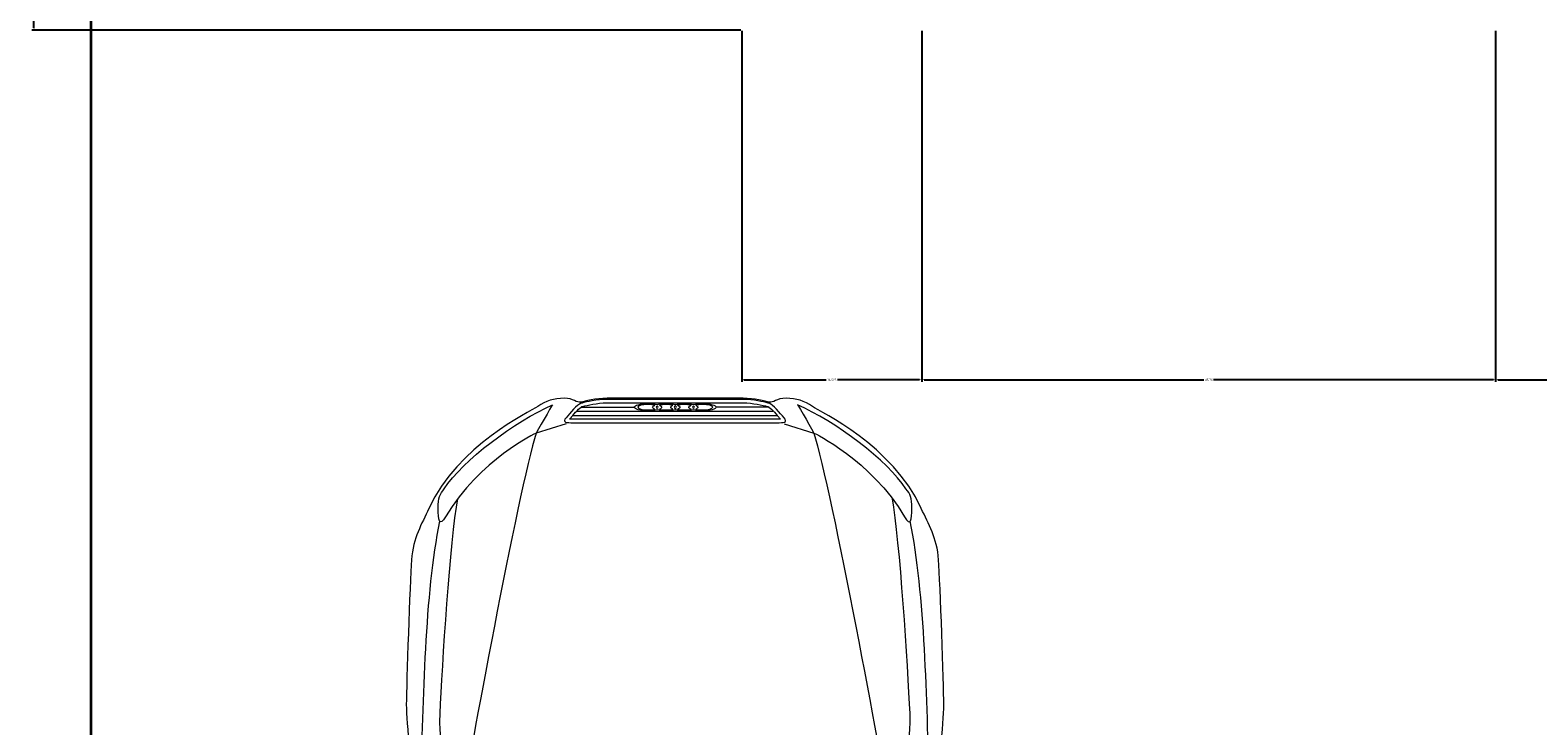
# Model space of a CAD drawing. Units: inches. Extents: x 1976 to 2558, y -977 to 2909.
# Tile 2 of 8: x 2050 to 2173, y 1970 to 2026. Entities that reach past the tile are written whole.
import ezdxf

# ---------------------------------------------------------------- set-up
doc = ezdxf.new("R2010")
doc.units = ezdxf.units.IN
for name, color, linetype, lineweight in [('A-ANNO-DIMS', 2, 'Continuous', 18), ('A-ANNO-TTLB', 7, 'Continuous', 35), ('AUDI', 7, 'Continuous', 18)]:
    doc.layers.add(name, color=color, linetype=linetype, lineweight=lineweight)
doc.styles.get("Standard").update_dxf_attribs({"font": 'arial.ttf'})
doc.dimstyles.get("Standard").update_dxf_attribs({"dimtxt": 0.18, "dimasz": 0.18, "dimexe": 0.18, "dimexo": 0.0625, "dimgap": 0.09, "dimtad": 0, "dimtih": 1, "dimtoh": 1, "dimdec": 4, "dimzin": 0, "dimdsep": 46, "dimtxsty": 'Standard', "dimcen": 0.09, "dimadec": 0, "dimazin": 0, "dimtfac": 1, "dimtdec": 4, "dimtofl": 0, "dimtmove": 0, "dimatfit": 3, "dimfxl": 1, "dimtolj": 1, "dimtzin": 0, "dimarcsym": 0})

# ---------------------------------------------------------------- blocks, each defined once
blk = doc.blocks.new('*D36')
at = {"layer": 'A-ANNO-DIMS', "color": 0, "lineweight": -2, "transparency": 16777216}
for p, q in [((2108.38, 2117.06), (2050.58, 2117.06)), ((2050.76, 2116.88), (2050.76, 2071.95)), ((2050.76, 2026.66), (2050.76, 2071.59)), ((2108.38, 2026.48), (2050.58, 2026.48))]:
    blk.add_line(p, q, dxfattribs=at)
at = {"layer": 'A-ANNO-DIMS', "color": 0, "transparency": 16777216}
for points in [[(2050.73, 2116.88), (2050.79, 2116.88), (2050.76, 2117.06)], [(2050.73, 2026.66), (2050.79, 2026.66), (2050.76, 2026.48)]]:
    blk.add_solid(points, dxfattribs=at)
at = {"layer": 'Defpoints', "color": 0, "transparency": 16777216}
for p in [(2108.44, 2117.06), (2050.76, 2026.48), (2108.44, 2026.48)]:
    blk.add_point(p, dxfattribs=at)
at = {"layer": 'A-ANNO-DIMS', "color": 0, "transparency": 16777216, "insert": (2050.76, 2071.77), "char_height": 0.18, "attachment_point": 5}
blk.add_mtext('\\A1;90.58', dxfattribs=at)
blk = doc.blocks.new('*D42')
at = {"layer": 'A-ANNO-DIMS', "color": 0, "lineweight": -2, "transparency": 16777216}
for p, q in [((2108.44, 2026.42), (2108.44, 1997.8)), ((2123.12, 2026.42), (2123.12, 1997.8)), ((2108.62, 1997.98), (2115.33, 1997.98)), ((2122.94, 1997.98), (2116.24, 1997.98))]:
    blk.add_line(p, q, dxfattribs=at)
at = {"layer": 'A-ANNO-DIMS', "color": 0, "transparency": 16777216}
for points in [[(2108.62, 1998.01), (2108.62, 1997.95), (2108.44, 1997.98)], [(2122.94, 1998.01), (2122.94, 1997.95), (2123.12, 1997.98)]]:
    blk.add_solid(points, dxfattribs=at)
at = {"layer": 'Defpoints', "color": 0, "transparency": 16777216}
for p in [(2108.44, 2026.48), (2123.12, 2026.48), (2108.44, 1997.98)]:
    blk.add_point(p, dxfattribs=at)
at = {"layer": 'A-ANNO-DIMS', "color": 0, "transparency": 16777216, "insert": (2115.78, 1997.98), "char_height": 0.18, "attachment_point": 5}
blk.add_mtext('\\A1;14.686', dxfattribs=at)
blk = doc.blocks.new('*D43')
at = {"layer": 'A-ANNO-DIMS', "color": 0, "lineweight": -2, "transparency": 16777216}
for p, q in [((2123.12, 2026.42), (2123.12, 1997.8)), ((2169.89, 2026.42), (2169.89, 1997.8)), ((2123.3, 1997.98), (2146.11, 1997.98)), ((2169.71, 1997.98), (2146.9, 1997.98))]:
    blk.add_line(p, q, dxfattribs=at)
at = {"layer": 'A-ANNO-DIMS', "color": 0, "transparency": 16777216}
for points in [[(2123.3, 1998.01), (2123.3, 1997.95), (2123.12, 1997.98)], [(2169.71, 1998.01), (2169.71, 1997.95), (2169.89, 1997.98)]]:
    blk.add_solid(points, dxfattribs=at)
at = {"layer": 'Defpoints', "color": 0, "transparency": 16777216}
for p in [(2123.12, 2026.48), (2169.89, 2026.48), (2123.12, 1997.98)]:
    blk.add_point(p, dxfattribs=at)
at = {"layer": 'A-ANNO-DIMS', "color": 0, "transparency": 16777216, "insert": (2146.51, 1997.98), "char_height": 0.18, "attachment_point": 5}
blk.add_mtext('\\A1;46.76', dxfattribs=at)
blk = doc.blocks.new('*D44')
at = {"layer": 'A-ANNO-DIMS', "color": 0, "lineweight": -2, "transparency": 16777216}
for p, q in [((2169.89, 2026.42), (2169.89, 1997.8)), ((2183.44, 2026.42), (2183.44, 1997.8)), ((2170.07, 1997.98), (2176.21, 1997.98)), ((2183.26, 1997.98), (2177.12, 1997.98))]:
    blk.add_line(p, q, dxfattribs=at)
at = {"layer": 'A-ANNO-DIMS', "color": 0, "transparency": 16777216}
for points in [[(2170.07, 1998.01), (2170.07, 1997.95), (2169.89, 1997.98)], [(2183.26, 1998.01), (2183.26, 1997.95), (2183.44, 1997.98)]]:
    blk.add_solid(points, dxfattribs=at)
at = {"layer": 'Defpoints', "color": 0, "transparency": 16777216}
for p in [(2169.89, 2026.48), (2183.44, 2026.48), (2169.89, 1997.98)]:
    blk.add_point(p, dxfattribs=at)
at = {"layer": 'A-ANNO-DIMS', "color": 0, "transparency": 16777216, "insert": (2176.66, 1997.98), "char_height": 0.18, "attachment_point": 5}
blk.add_mtext('\\A1;13.552', dxfattribs=at)

msp = doc.modelspace()

# ---------------------------------------------------------------- linework, layer by layer
at = {"layer": 'A-ANNO-TTLB'}
msp.add_lwpolyline([(2055.4343, 2428.9091), (2450.0007, 2428.9091), (2450.0007, 1815.3916), (2055.4343, 1815.3916)], close=True, dxfattribs=at)
at = {"layer": 'AUDI'}
for points, knots in [([(2103.0114, 1886.9558), (2086.9517, 1887.1313), (2084.6199, 1892.5316), (2083.6345, 1896.09), (2083.6345, 1896.09), (2082.9917, 1898.1907), (2082.4777, 1899.8626), (2082.2206, 1900.7202), (2082.2206, 1900.7202), (2081.9634, 1901.5775), (2081.4067, 1904.1927), (2081.3636, 1906.3792), (2081.3636, 1906.3792), (2081.3206, 1908.5657), (2081.1085, 1921.6021), (2081.1085, 1925.2), (2081.1085, 1925.2), (2081.1085, 1928.7977), (2081.1085, 1945.653), (2081.1085, 1948.0508), (2081.1085, 1948.0508), (2081.1085, 1950.4484), (2081.6208, 1960.012), (2081.6208, 1963.0558), (2081.6208, 1963.0558), (2081.6208, 1966.0998), (2081.1085, 1969.9188), (2081.1085, 1971.5013), (2081.1085, 1971.5013), (2081.1085, 1973.084), (2081.4064, 1981.4476), (2081.535, 1983.2912), (2081.535, 1983.2912), (2081.6638, 1985.1347), (2082.3541, 1986.1803), (2082.9493, 1987.4927), (2082.9493, 1987.4927), (2085.2631, 1992.5941), (2091.1759, 1995.3806), (2091.8187, 1995.8094), (2091.8187, 1995.8094), (2092.4614, 1996.2383), (2093.1437, 1996.4712), (2093.9611, 1996.4712), (2093.9611, 1996.4712), (2094.7784, 1996.4712), (2094.9894, 1996.0668), (2095.3323, 1996.1525), (2095.3323, 1996.1525), (2095.6751, 1996.2383), (2096.5292, 1996.4712), (2097.4749, 1996.4712), (2097.4749, 1996.4712), (2098.4207, 1996.4712), (2103.0114, 1996.4712), (2103.0114, 1996.4712), (2103.0114, 1996.4712), (2103.0114, 1996.4712), (2107.6023, 1996.4712), (2108.548, 1996.4712), (2108.548, 1996.4712), (2109.4939, 1996.4712), (2110.3478, 1996.2383), (2110.6907, 1996.1525), (2110.6907, 1996.1525), (2111.0335, 1996.0668), (2111.2446, 1996.4712), (2112.0619, 1996.4712), (2112.0619, 1996.4712), (2112.8792, 1996.4712), (2113.5616, 1996.2383), (2114.2043, 1995.8094), (2114.2043, 1995.8094), (2114.847, 1995.3807), (2120.7599, 1992.5941), (2123.0737, 1987.4927), (2123.0737, 1987.4927), (2123.6688, 1986.1803), (2124.3592, 1985.1347), (2124.4878, 1983.2912), (2124.4878, 1983.2912), (2124.6166, 1981.4477), (2124.9145, 1973.0839), (2124.9145, 1971.5013), (2124.9145, 1971.5013), (2124.9145, 1969.9189), (2124.4021, 1966.0998), (2124.4021, 1963.0558), (2124.4021, 1963.0558), (2124.4021, 1960.012), (2124.9145, 1950.4484), (2124.9145, 1948.0508), (2124.9145, 1948.0508), (2124.9145, 1945.653), (2124.9145, 1928.7977), (2124.9145, 1925.2), (2124.9145, 1925.2), (2124.9145, 1921.6021), (2124.7023, 1908.5656), (2124.6593, 1906.3792), (2124.6593, 1906.3792), (2124.6164, 1904.1927), (2124.0596, 1901.5775), (2123.8024, 1900.7202), (2123.8024, 1900.7202), (2123.5452, 1899.8626), (2123.0312, 1898.1907), (2122.3885, 1896.09), (2122.3885, 1896.09), (2121.4031, 1892.5316), (2119.0712, 1887.1313), (2103.0114, 1886.9558)], [0, 0, 0, 0, 0.03571429, 0.03571429, 0.03571429, 0.0357143, 0.07142857, 0.07142857, 0.07142857, 0.07142858, 0.10714286, 0.10714286, 0.10714286, 0.10714287, 0.14285714, 0.14285714, 0.14285714, 0.14285715, 0.17857143, 0.17857143, 0.17857143, 0.17857144, 0.21428571, 0.21428571, 0.21428571, 0.21428572, 0.25, 0.25, 0.25, 0.25000001, 0.28571429, 0.28571429, 0.28571429, 0.2857143, 0.32142857, 0.32142857, 0.32142857, 0.32142858, 0.35714286, 0.35714286, 0.35714286, 0.35714287, 0.39285714, 0.39285714, 0.39285714, 0.39285715, 0.42857143, 0.42857143, 0.42857143, 0.42857144, 0.46428571, 0.46428571, 0.46428571, 0.46428572, 0.5, 0.5, 0.5, 0.50000001, 0.53571429, 0.53571429, 0.53571429, 0.5357143, 0.57142857, 0.57142857, 0.57142857, 0.57142858, 0.60714286, 0.60714286, 0.60714286, 0.60714287, 0.64285714, 0.64285714, 0.64285714, 0.64285715, 0.67857143, 0.67857143, 0.67857143, 0.67857144, 0.71428571, 0.71428571, 0.71428571, 0.71428572, 0.75, 0.75, 0.75, 0.75000001, 0.78571429, 0.78571429, 0.78571429, 0.7857143, 0.82142857, 0.82142857, 0.82142857, 0.82142858, 0.85714286, 0.85714286, 0.85714286, 0.85714287, 0.89285714, 0.89285714, 0.89285714, 0.89285715, 0.92857143, 0.92857143, 0.92857143, 0.92857144, 0.96428571, 0.96428571, 0.96428571, 0.96428572, 1, 1, 1, 1]), ([(2083.7046, 1987.5032), (2083.7046, 1986.5496), (2083.814, 1985.971), (2084.3029, 1986.7989), (2084.3029, 1986.7989), (2087.0487, 1991.448), (2091.6954, 1993.6314), (2091.6954, 1993.6314), (2091.6954, 1993.6314), (2091.6954, 1993.6315), (2092.9543, 1995.8893), (2093.0331, 1995.9208), (2093.0331, 1995.9208), (2089.9674, 1994.6232), (2085.6616, 1991.3535), (2084.1974, 1989.0883), (2084.1974, 1989.0883), (2083.8454, 1988.6304), (2083.7046, 1988.4021), (2083.7046, 1987.5032)], [0, 0, 0, 0, 0.2, 0.2, 0.2, 0.20000001, 0.4, 0.4, 0.4, 0.40000001, 0.6, 0.6, 0.6, 0.60000001, 0.8, 0.8, 0.8, 0.80000001, 1, 1, 1, 1]), ([(2083.7046, 1987.5032), (2083.7046, 1986.5496), (2083.814, 1985.971), (2084.3029, 1986.7989), (2084.3029, 1986.7989), (2087.0487, 1991.448), (2091.6954, 1993.6314), (2091.6954, 1993.6314), (2091.6954, 1993.6314), (2091.6954, 1993.6314), (2092.9543, 1995.8893), (2093.0331, 1995.9208), (2093.0331, 1995.9208), (2089.9674, 1994.6232), (2085.6616, 1991.3535), (2084.1974, 1989.0883), (2084.1974, 1989.0883), (2083.8454, 1988.6304), (2083.7046, 1988.4021), (2083.7046, 1987.5032)], [0, 0, 0, 0, 0.2, 0.2, 0.2, 0.20000001, 0.4, 0.4, 0.4, 0.40000001, 0.6, 0.6, 0.6, 0.60000001, 0.8, 0.8, 0.8, 0.80000001, 1, 1, 1, 1]), ([(2103.1016, 1996.3775), (2103.1016, 1996.3775), (2108.548, 1996.3775), (2108.548, 1996.3775), (2108.548, 1996.3775), (2109.4216, 1996.3775), (2110.2145, 1996.1765), (2110.5954, 1996.08), (2110.5954, 1996.08), (2110.5954, 1996.08), (2110.6679, 1996.0617), (2110.6679, 1996.0617), (2110.6679, 1996.0617), (2111.0143, 1995.9511), (2111.55, 1995.2541), (2111.8895, 1994.8788), (2111.8895, 1994.8788), (2112.2289, 1994.5035), (2111.8895, 1994.4678), (2111.2821, 1994.4678), (2111.2821, 1994.4678), (2110.6748, 1994.4678), (2103.0114, 1994.4678), (2103.0114, 1994.4678), (2103.0114, 1994.4678), (2103.0114, 1994.4678), (2095.3482, 1994.4678), (2094.7408, 1994.4678), (2094.7408, 1994.4678), (2094.1335, 1994.4678), (2093.794, 1994.5035), (2094.1335, 1994.8788), (2094.1335, 1994.8788), (2094.4729, 1995.2541), (2095.0087, 1995.9511), (2095.355, 1996.0617), (2095.355, 1996.0617), (2095.355, 1996.0617), (2095.4275, 1996.0801), (2095.4275, 1996.0801), (2095.4275, 1996.0801), (2095.8085, 1996.1765), (2096.6014, 1996.3774), (2097.4749, 1996.3774), (2097.4749, 1996.3774), (2097.4749, 1996.3774), (2102.9214, 1996.3775), (2102.9214, 1996.3775), (2102.9214, 1996.3775), (2102.9214, 1996.3775), (2103.1016, 1996.3775), (2103.1016, 1996.3775)], [0, 0, 0, 0, 0.07692308, 0.07692308, 0.07692308, 0.07692309, 0.15384615, 0.15384615, 0.15384615, 0.15384616, 0.23076923, 0.23076923, 0.23076923, 0.23076924, 0.30769231, 0.30769231, 0.30769231, 0.30769232, 0.38461538, 0.38461538, 0.38461538, 0.38461539, 0.46153846, 0.46153846, 0.46153846, 0.46153847, 0.53846154, 0.53846154, 0.53846154, 0.53846155, 0.61538462, 0.61538462, 0.61538462, 0.61538463, 0.69230769, 0.69230769, 0.69230769, 0.6923077, 0.76923077, 0.76923077, 0.76923077, 0.76923078, 0.84615385, 0.84615385, 0.84615385, 0.84615386, 0.92307692, 0.92307692, 0.92307692, 0.92307693, 1, 1, 1, 1]), ([(2094.7408, 1994.7516), (2094.7408, 1994.7516), (2094.7408, 1994.7516), (2094.7408, 1994.7516), (2094.7408, 1994.7516), (2094.7408, 1994.7516), (2111.2821, 1994.7516), (2111.2821, 1994.7516), (2111.2821, 1994.7516), (2111.4218, 1994.7516), (2111.5292, 1994.755), (2111.6164, 1994.7604), (2111.6164, 1994.7604), (2111.5495, 1994.8371), (2111.4462, 1994.9552), (2111.4462, 1994.9552), (2111.4462, 1994.9552), (2111.1976, 1995.2442), (2110.7818, 1995.7269), (2110.5822, 1995.7909), (2110.5822, 1995.7909), (2110.5822, 1995.7909), (2110.5261, 1995.8048), (2110.5261, 1995.8048), (2110.5261, 1995.8048), (2110.1549, 1995.8989), (2109.3854, 1996.0939), (2108.548, 1996.0939), (2108.548, 1996.0939), (2108.548, 1996.0939), (2097.4749, 1996.094), (2097.4749, 1996.094), (2097.4749, 1996.094), (2096.6375, 1996.094), (2095.8681, 1995.8988), (2095.4981, 1995.8053), (2095.4981, 1995.8053), (2095.4981, 1995.8053), (2095.4244, 1995.7865), (2095.4244, 1995.7865), (2095.4244, 1995.7865), (2095.2417, 1995.7279), (2094.8256, 1995.2441), (2094.5767, 1994.9552), (2094.5767, 1994.9552), (2094.5767, 1994.9552), (2094.4737, 1994.8371), (2094.4065, 1994.7604), (2094.4065, 1994.7604), (2094.4939, 1994.755), (2094.6011, 1994.7516), (2094.7408, 1994.7516)], [0, 0, 0, 0, 0.07692308, 0.07692308, 0.07692308, 0.07692309, 0.15384615, 0.15384615, 0.15384615, 0.15384616, 0.23076923, 0.23076923, 0.23076923, 0.23076924, 0.30769231, 0.30769231, 0.30769231, 0.30769232, 0.38461538, 0.38461538, 0.38461538, 0.38461539, 0.46153846, 0.46153846, 0.46153846, 0.46153847, 0.53846154, 0.53846154, 0.53846154, 0.53846155, 0.61538462, 0.61538462, 0.61538462, 0.61538463, 0.69230769, 0.69230769, 0.69230769, 0.6923077, 0.76923077, 0.76923077, 0.76923077, 0.76923078, 0.84615385, 0.84615385, 0.84615385, 0.84615386, 0.92307692, 0.92307692, 0.92307692, 0.92307693, 1, 1, 1, 1]), ([(2100.8027, 1995.4423), (2101.0908, 1995.4423), (2101.3428, 1995.4713), (2101.5407, 1995.5201), (2101.5407, 1995.5201), (2101.7389, 1995.4713), (2102.009, 1995.4422), (2102.2972, 1995.4422), (2102.2972, 1995.4422), (2102.5851, 1995.4423), (2102.8371, 1995.4713), (2103.0352, 1995.5152), (2103.0352, 1995.5152), (2103.2149, 1995.4713), (2103.4854, 1995.4422), (2103.7553, 1995.4422), (2103.7553, 1995.4422), (2104.0435, 1995.4423), (2104.3136, 1995.4713), (2104.5116, 1995.5201), (2104.5116, 1995.5201), (2104.7097, 1995.4713), (2104.9617, 1995.4422), (2105.2496, 1995.4422), (2105.2496, 1995.4422), (2105.8621, 1995.4423), (2106.3661, 1995.5733), (2106.3661, 1995.7381), (2106.3661, 1995.7381), (2106.3661, 1995.8981), (2105.8621, 1996.0344), (2105.2496, 1996.0344), (2105.2496, 1996.0344), (2104.9617, 1996.0344), (2104.7097, 1996.0004), (2104.5116, 1995.9565), (2104.5116, 1995.9565), (2104.3136, 1996.0005), (2104.0435, 1996.0344), (2103.7553, 1996.0344), (2103.7553, 1996.0344), (2103.4854, 1996.0344), (2103.2149, 1996.0053), (2103.0352, 1995.9565), (2103.0352, 1995.9565), (2102.8371, 1996.0054), (2102.5851, 1996.0344), (2102.2972, 1996.0344), (2102.2972, 1996.0344), (2101.9763, 1996.0344), (2101.6291, 1995.9762), (2101.5407, 1995.9565), (2101.5407, 1995.9565), (2101.3428, 1996.0005), (2101.0908, 1996.0344), (2100.8027, 1996.0344), (2100.8027, 1996.0344), (2100.1905, 1996.0344), (2099.6862, 1995.898), (2099.6862, 1995.7381), (2099.6862, 1995.7381), (2099.6862, 1995.5733), (2100.1905, 1995.4422), (2100.8027, 1995.4423)], [0, 0, 0, 0, 0.0625, 0.0625, 0.0625, 0.06250001, 0.125, 0.125, 0.125, 0.12500001, 0.1875, 0.1875, 0.1875, 0.18750001, 0.25, 0.25, 0.25, 0.25000001, 0.3125, 0.3125, 0.3125, 0.31250001, 0.375, 0.375, 0.375, 0.37500001, 0.4375, 0.4375, 0.4375, 0.43750001, 0.5, 0.5, 0.5, 0.50000001, 0.5625, 0.5625, 0.5625, 0.56250001, 0.625, 0.625, 0.625, 0.62500001, 0.6875, 0.6875, 0.6875, 0.68750001, 0.75, 0.75, 0.75, 0.75000001, 0.8125, 0.8125, 0.8125, 0.81250001, 0.875, 0.875, 0.875, 0.87500001, 0.9375, 0.9375, 0.9375, 0.93750001, 1, 1, 1, 1]), ([(2100.8027, 1995.4423), (2101.0908, 1995.4423), (2101.3428, 1995.4713), (2101.5407, 1995.5201), (2101.5407, 1995.5201), (2101.7389, 1995.4713), (2102.009, 1995.4422), (2102.2972, 1995.4422), (2102.2972, 1995.4422), (2102.5851, 1995.4422), (2102.8371, 1995.4713), (2103.0352, 1995.5152), (2103.0352, 1995.5152), (2103.2149, 1995.4713), (2103.4854, 1995.4422), (2103.7553, 1995.4422), (2103.7553, 1995.4422), (2104.0435, 1995.4422), (2104.3136, 1995.4713), (2104.5116, 1995.5201), (2104.5116, 1995.5201), (2104.7097, 1995.4713), (2104.9617, 1995.4422), (2105.2496, 1995.4422), (2105.2496, 1995.4422), (2105.8621, 1995.4422), (2106.3661, 1995.5733), (2106.3661, 1995.7381), (2106.3661, 1995.7381), (2106.3661, 1995.8981), (2105.8621, 1996.0344), (2105.2496, 1996.0344), (2105.2496, 1996.0344), (2104.9617, 1996.0344), (2104.7097, 1996.0004), (2104.5116, 1995.9565), (2104.5116, 1995.9565), (2104.3136, 1996.0005), (2104.0435, 1996.0344), (2103.7553, 1996.0344), (2103.7553, 1996.0344), (2103.4854, 1996.0344), (2103.2149, 1996.0053), (2103.0352, 1995.9565), (2103.0352, 1995.9565), (2102.8371, 1996.0054), (2102.5851, 1996.0344), (2102.2972, 1996.0344), (2102.2972, 1996.0344), (2101.9763, 1996.0344), (2101.6291, 1995.9762), (2101.5407, 1995.9565), (2101.5407, 1995.9565), (2101.3428, 1996.0005), (2101.0908, 1996.0344), (2100.8027, 1996.0344), (2100.8027, 1996.0344), (2100.1905, 1996.0344), (2099.6862, 1995.898), (2099.6862, 1995.7381), (2099.6862, 1995.7381), (2099.6862, 1995.5733), (2100.1905, 1995.4423), (2100.8027, 1995.4423)], [0, 0, 0, 0, 0.0625, 0.0625, 0.0625, 0.06250001, 0.125, 0.125, 0.125, 0.12500001, 0.1875, 0.1875, 0.1875, 0.18750001, 0.25, 0.25, 0.25, 0.25000001, 0.3125, 0.3125, 0.3125, 0.31250001, 0.375, 0.375, 0.375, 0.37500001, 0.4375, 0.4375, 0.4375, 0.43750001, 0.5, 0.5, 0.5, 0.50000001, 0.5625, 0.5625, 0.5625, 0.56250001, 0.625, 0.625, 0.625, 0.62500001, 0.6875, 0.6875, 0.6875, 0.68750001, 0.75, 0.75, 0.75, 0.75000001, 0.8125, 0.8125, 0.8125, 0.81250001, 0.875, 0.875, 0.875, 0.87500001, 0.9375, 0.9375, 0.9375, 0.93750001, 1, 1, 1, 1]), ([(2100.8027, 1995.9565), (2101.0185, 1995.9565), (2101.2169, 1995.9372), (2101.3609, 1995.898), (2101.3609, 1995.898), (2101.2527, 1995.8498), (2101.1807, 1995.7965), (2101.1807, 1995.7381), (2101.1807, 1995.7381), (2101.1807, 1995.6752), (2101.2527, 1995.6219), (2101.3609, 1995.5733), (2101.3609, 1995.5733), (2101.2169, 1995.5394), (2101.0185, 1995.5152), (2100.8027, 1995.5152), (2100.8027, 1995.5152), (2100.3345, 1995.5152), (2099.9743, 1995.6121), (2099.9743, 1995.7381), (2099.9743, 1995.7381), (2099.9743, 1995.8595), (2100.3345, 1995.9565), (2100.8027, 1995.9565)], [0, 0, 0, 0, 0.16666667, 0.16666667, 0.16666667, 0.16666668, 0.33333333, 0.33333333, 0.33333333, 0.33333334, 0.5, 0.5, 0.5, 0.50000001, 0.66666667, 0.66666667, 0.66666667, 0.66666668, 0.83333333, 0.83333333, 0.83333333, 0.83333334, 1, 1, 1, 1]), ([(2101.631, 1995.7382), (2101.631, 1995.6994), (2101.5949, 1995.6702), (2101.5407, 1995.6412), (2101.5407, 1995.6412), (2101.4869, 1995.6703), (2101.4689, 1995.6993), (2101.4689, 1995.7381), (2101.4689, 1995.7381), (2101.4689, 1995.7724), (2101.4869, 1995.806), (2101.5407, 1995.8353), (2101.5407, 1995.8353), (2101.5949, 1995.806), (2101.631, 1995.7723), (2101.631, 1995.7382)], [0, 0, 0, 0, 0.25, 0.25, 0.25, 0.25000001, 0.5, 0.5, 0.5, 0.50000001, 0.75, 0.75, 0.75, 0.75000001, 1, 1, 1, 1]), ([(2102.8371, 1995.903), (2102.7289, 1995.8547), (2102.6572, 1995.7965), (2102.6572, 1995.7381), (2102.6572, 1995.7381), (2102.6572, 1995.6752), (2102.7289, 1995.617), (2102.8371, 1995.5684), (2102.8371, 1995.5684), (2102.6933, 1995.5345), (2102.5131, 1995.5152), (2102.2972, 1995.5152), (2102.2972, 1995.5152), (2102.0808, 1995.5152), (2101.883, 1995.5394), (2101.7389, 1995.5733), (2101.7389, 1995.5733), (2101.8469, 1995.622), (2101.9189, 1995.6751), (2101.9189, 1995.7381), (2101.9189, 1995.7381), (2101.9189, 1995.7965), (2101.8469, 1995.8498), (2101.7389, 1995.898), (2101.7389, 1995.898), (2101.883, 1995.9372), (2102.0808, 1995.9565), (2102.2972, 1995.9565), (2102.2972, 1995.9565), (2102.5131, 1995.9565), (2102.6933, 1995.9372), (2102.8371, 1995.903)], [0, 0, 0, 0, 0.125, 0.125, 0.125, 0.12500001, 0.25, 0.25, 0.25, 0.25000001, 0.375, 0.375, 0.375, 0.37500001, 0.5, 0.5, 0.5, 0.50000001, 0.625, 0.625, 0.625, 0.62500001, 0.75, 0.75, 0.75, 0.75000001, 0.875, 0.875, 0.875, 0.87500001, 1, 1, 1, 1]), ([(2103.125, 1995.7382), (2103.125, 1995.6994), (2103.0893, 1995.6653), (2103.0352, 1995.6314), (2103.0352, 1995.6314), (2102.9631, 1995.6654), (2102.9272, 1995.6993), (2102.9272, 1995.7381), (2102.9272, 1995.7381), (2102.9272, 1995.7724), (2102.9631, 1995.8109), (2103.0352, 1995.8402), (2103.0352, 1995.8402), (2103.0893, 1995.811), (2103.125, 1995.7723), (2103.125, 1995.7382)], [0, 0, 0, 0, 0.25, 0.25, 0.25, 0.25000001, 0.5, 0.5, 0.5, 0.50000001, 0.75, 0.75, 0.75, 0.75000001, 1, 1, 1, 1]), ([(2104.3314, 1995.8981), (2104.2053, 1995.8498), (2104.1336, 1995.7965), (2104.1336, 1995.7381), (2104.1336, 1995.7381), (2104.1336, 1995.6752), (2104.2053, 1995.6219), (2104.3314, 1995.5733), (2104.3314, 1995.5733), (2104.1695, 1995.5394), (2103.9714, 1995.5152), (2103.7553, 1995.5152), (2103.7553, 1995.5152), (2103.5573, 1995.5152), (2103.3592, 1995.5345), (2103.2149, 1995.5684), (2103.2149, 1995.5684), (2103.3414, 1995.6171), (2103.4132, 1995.6751), (2103.4132, 1995.7381), (2103.4132, 1995.7381), (2103.4132, 1995.7965), (2103.3414, 1995.8546), (2103.2149, 1995.9029), (2103.2149, 1995.9029), (2103.3592, 1995.9372), (2103.5573, 1995.9565), (2103.7553, 1995.9565), (2103.7553, 1995.9565), (2103.9714, 1995.9565), (2104.1695, 1995.9372), (2104.3314, 1995.8981)], [0, 0, 0, 0, 0.125, 0.125, 0.125, 0.12500001, 0.25, 0.25, 0.25, 0.25000001, 0.375, 0.375, 0.375, 0.37500001, 0.5, 0.5, 0.5, 0.50000001, 0.625, 0.625, 0.625, 0.62500001, 0.75, 0.75, 0.75, 0.75000001, 0.875, 0.875, 0.875, 0.87500001, 1, 1, 1, 1]), ([(2104.6014, 1995.7382), (2104.6014, 1995.6994), (2104.5656, 1995.6702), (2104.5116, 1995.6412), (2104.5116, 1995.6412), (2104.4574, 1995.6703), (2104.4215, 1995.6993), (2104.4215, 1995.7381), (2104.4215, 1995.7381), (2104.4215, 1995.7724), (2104.4574, 1995.806), (2104.5116, 1995.8353), (2104.5116, 1995.8353), (2104.5656, 1995.806), (2104.6014, 1995.7723), (2104.6014, 1995.7382)], [0, 0, 0, 0, 0.25, 0.25, 0.25, 0.25000001, 0.5, 0.5, 0.5, 0.50000001, 0.75, 0.75, 0.75, 0.75000001, 1, 1, 1, 1]), ([(2106.0779, 1995.7382), (2106.0779, 1995.6122), (2105.718, 1995.5152), (2105.2496, 1995.5152), (2105.2496, 1995.5152), (2105.0337, 1995.5152), (2104.8356, 1995.5394), (2104.6916, 1995.5733), (2104.6916, 1995.5733), (2104.7998, 1995.622), (2104.8716, 1995.6751), (2104.8716, 1995.7381), (2104.8716, 1995.7381), (2104.8716, 1995.7965), (2104.7998, 1995.8498), (2104.6916, 1995.898), (2104.6916, 1995.898), (2104.8356, 1995.9372), (2105.0337, 1995.9565), (2105.2496, 1995.9565), (2105.2496, 1995.9565), (2105.718, 1995.9565), (2106.0779, 1995.8595), (2106.0779, 1995.7382)], [0, 0, 0, 0, 0.16666667, 0.16666667, 0.16666667, 0.16666668, 0.33333333, 0.33333333, 0.33333333, 0.33333334, 0.5, 0.5, 0.5, 0.50000001, 0.66666667, 0.66666667, 0.66666667, 0.66666668, 0.83333333, 0.83333333, 0.83333333, 0.83333334, 1, 1, 1, 1]), ([(2122.3184, 1987.5032), (2122.3184, 1986.5496), (2122.209, 1985.971), (2121.7201, 1986.7989), (2121.7201, 1986.7989), (2118.9743, 1991.448), (2114.3276, 1993.6314), (2114.3276, 1993.6314), (2114.3276, 1993.6314), (2114.3276, 1993.6315), (2113.0687, 1995.8893), (2112.9898, 1995.9208), (2112.9898, 1995.9208), (2116.0555, 1994.6232), (2120.3613, 1991.3535), (2121.8256, 1989.0883), (2121.8256, 1989.0883), (2122.1774, 1988.6304), (2122.3184, 1988.4021), (2122.3184, 1987.5032)], [0, 0, 0, 0, 0.2, 0.2, 0.2, 0.20000001, 0.4, 0.4, 0.4, 0.40000001, 0.6, 0.6, 0.6, 0.60000001, 0.8, 0.8, 0.8, 0.80000001, 1, 1, 1, 1]), ([(2122.3184, 1987.5032), (2122.3184, 1986.5496), (2122.209, 1985.971), (2121.7201, 1986.7989), (2121.7201, 1986.7989), (2118.9743, 1991.448), (2114.3276, 1993.6314), (2114.3276, 1993.6314), (2114.3276, 1993.6314), (2114.3276, 1993.6314), (2113.0687, 1995.8893), (2112.9898, 1995.9208), (2112.9898, 1995.9208), (2116.0555, 1994.6232), (2120.3613, 1991.3535), (2121.8256, 1989.0883), (2121.8256, 1989.0883), (2122.1774, 1988.6304), (2122.3184, 1988.4021), (2122.3184, 1987.5032)], [0, 0, 0, 0, 0.2, 0.2, 0.2, 0.20000001, 0.4, 0.4, 0.4, 0.40000001, 0.6, 0.6, 0.6, 0.60000001, 0.8, 0.8, 0.8, 0.80000001, 1, 1, 1, 1]), ([(2085.7492, 1964.0106), (2085.2492, 1965.0114), (2083.6975, 1967.0084), (2083.8628, 1970.7823), (2083.8628, 1970.7823), (2084.0282, 1974.5563), (2084.6983, 1984.9688), (2085.2995, 1988.2814)], [0, 0, 0, 0, 0.5, 0.5, 0.5, 0.50000001, 1, 1, 1, 1]), ([(2120.2736, 1964.0106), (2120.7738, 1965.0114), (2122.3255, 1967.0084), (2122.1602, 1970.7823), (2122.1602, 1970.7823), (2121.9948, 1974.5563), (2121.3247, 1984.9688), (2120.7235, 1988.2814)], [0, 0, 0, 0, 0.5, 0.5, 0.5, 0.50000001, 1, 1, 1, 1]), ([(2084.3876, 1896.043), (2083.5808, 1900.0799), (2082.7216, 1908.2552), (2082.5749, 1916.7694), (2082.5749, 1916.7694), (2082.4281, 1925.2835), (2082.0616, 1958.0186), (2082.2816, 1964.9178), (2082.2816, 1964.9178), (2082.5016, 1971.8171), (2082.6247, 1980.5207), (2083.8469, 1986.4445)], [0, 0, 0, 0, 0.33333333, 0.33333333, 0.33333333, 0.33333334, 0.66666667, 0.66666667, 0.66666667, 0.66666668, 1, 1, 1, 1]), ([(2121.6353, 1896.043), (2122.4422, 1900.0799), (2123.3013, 1908.2552), (2123.448, 1916.7694), (2123.448, 1916.7694), (2123.5948, 1925.2835), (2123.9614, 1958.0186), (2123.7414, 1964.9178), (2123.7414, 1964.9178), (2123.5213, 1971.8171), (2123.3982, 1980.5207), (2122.176, 1986.4445)], [0, 0, 0, 0, 0.33333333, 0.33333333, 0.33333333, 0.33333334, 0.66666667, 0.66666667, 0.66666667, 0.66666668, 1, 1, 1, 1])]:
    msp.add_open_spline(points, degree=3, knots=knots, dxfattribs=at)
for points in [[(2095.3548, 1995.7506), (2095.3548, 1995.7506), (2099.6862, 1995.7506), (2099.6862, 1995.7506)], [(2110.6682, 1995.7506), (2110.6682, 1995.7506), (2106.3368, 1995.7506), (2106.3368, 1995.7506)], [(2094.1278, 1994.3789), (2094.1278, 1994.3789), (2091.6954, 1993.6315), (2091.6954, 1993.6315)], [(2094.6685, 1995.0618), (2094.6685, 1995.0618), (2111.3349, 1995.0618), (2111.3349, 1995.0618)], [(2094.9845, 1995.4136), (2094.9845, 1995.4136), (2110.992, 1995.4136), (2110.992, 1995.4136)], [(2111.8951, 1994.3789), (2111.8951, 1994.3789), (2114.3276, 1993.6315), (2114.3276, 1993.6315)], [(2091.6954, 1993.6315), (2090.2812, 1989.1303), (2085.9918, 1966.0704), (2085.7417, 1963.8187)], [(2114.3276, 1993.6315), (2115.7417, 1989.1303), (2120.0311, 1966.0704), (2120.2812, 1963.8187)]]:
    msp.add_open_spline(points, degree=3, dxfattribs=at)

# ---------------------------------------------------------------- dimensions: what is measured, and where the dimension line sits
at = {"layer": 'A-ANNO-DIMS'}
for base, p1, p2, angle, override, picture, middle in [((2050.7562, 2026.4789), (2108.4385, 2117.0569), (2108.4385, 2026.4789), 90, {"dimdec": 2, "dimlfac": 1, "dimrnd": 0, "dimzin": 0, "dimdsep": 46, "dimlunit": 2}, '*D36', (2050.7562, 2071.7679)), ((2108.4385, 1997.9789), (2123.1248, 2026.4789), (2108.4385, 2026.4789), 180, {"dimdec": 3, "dimlfac": 1, "dimrnd": 0, "dimzin": 0, "dimdsep": 46, "dimlunit": 2}, '*D42', (2115.7816, 1997.9789)), ((2123.1248, 1997.9789), (2169.8866, 2026.4789), (2123.1248, 2026.4789), 180, {"dimdec": 2, "dimlfac": 1, "dimrnd": 0, "dimzin": 0, "dimdsep": 46, "dimlunit": 2}, '*D43', (2146.5057, 1997.9789)), ((2169.8866, 1997.9789), (2183.4385, 2026.4789), (2169.8866, 2026.4789), 180, {"dimdec": 3, "dimlfac": 1, "dimrnd": 0, "dimzin": 0, "dimdsep": 46, "dimlunit": 2}, '*D44', (2176.6625, 1997.9789))]:
    dim = msp.add_linear_dim(base=base, p1=p1, p2=p2, angle=angle, dimstyle='Standard', override=override, dxfattribs=at)
    dim.commit()
    dim.dimension.update_dxf_attribs({"geometry": picture, "text_midpoint": middle})

doc.saveas('drawing.dxf')
